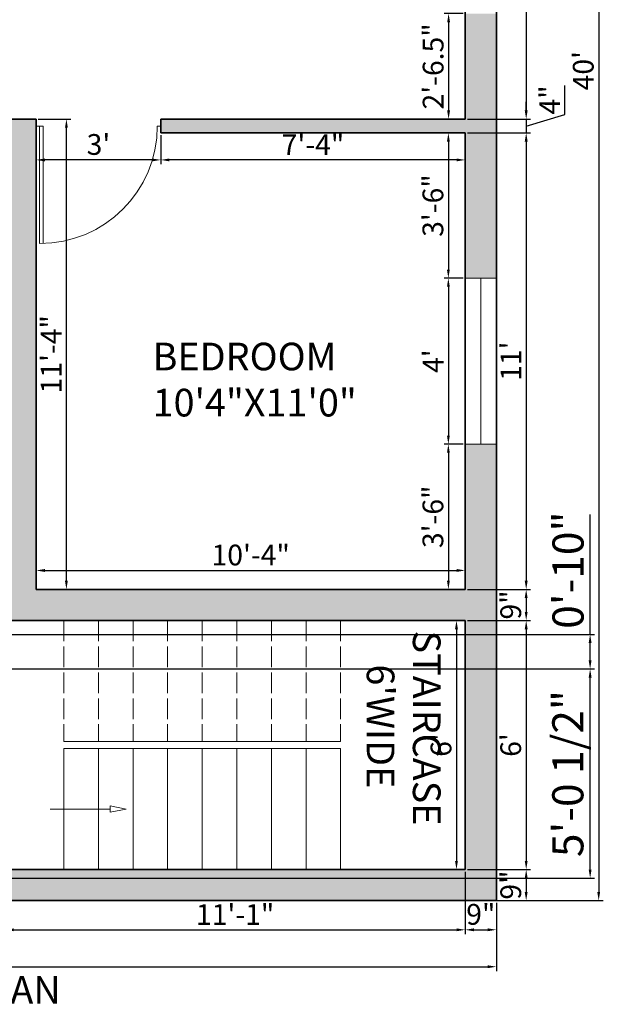
# Model space of a CAD drawing. Units: inches. Extents: x 3592 to 4861, y 1650 to 2243.
# Tile 28 of 30: x 4688 to 4861, y 1655 to 1940. Entities that reach past the tile are written whole.
import ezdxf

# ---------------------------------------------------------------- set-up
doc = ezdxf.new("R2010")
doc.units = ezdxf.units.IN
doc.linetypes.add('ACAD_ISO02W100', pattern=[15, 12, -3])
for name, color, linetype, lineweight in [('A-ANNO-DIMS', 2, 'Continuous', 13), ('A-ANNO-SYMB', 7, 'Continuous', 18), ('A-ANNO-TEXT', 7, 'Continuous', 25), ('A-AREA-IDEN', 7, 'Continuous', 18), ('A-DOOR', 3, 'Continuous', 20), ('A-FLOR-STRS', 7, 'Continuous', 18), ('A-FLOR-STRS-OVHD', 8, 'ACAD_ISO02W100', 13), ('A-GLAZ', 4, 'Continuous', 18), ('A-WALL', 7, 'Continuous', 35)]:
    doc.layers.add(name, color=color, linetype=linetype, lineweight=lineweight)
doc.layers.add('A-WALL-PATT', color=252, linetype='Continuous', lineweight=13, true_color=0x939598)
doc.styles.get("Standard").update_dxf_attribs({"font": 'arial.ttf'})
doc.dimstyles.new('ISO-25', dxfattribs={"dimtxt": 9, "dimasz": 2.5, "dimexe": 1.25, "dimexo": 0.625, "dimtad": 1, "dimlunit": 3, "dimtxsty": 'Standard', "dimcen": 2.5, "dimadec": 0, "dimazin": 0, "dimtfac": 1, "dimtmove": 0, "dimatfit": 3, "dimfxl": 1, "dimarcsym": 0})

# ---------------------------------------------------------------- blocks, each defined once
blk = doc.blocks.new('1')
for p, q in [((3628.27, 1890.86), (3628.27, 1924.86)), ((3629.27, 1890.86), (3629.27, 1924.86)), ((3627.27, 1890.86), (3629.27, 1890.86)), ((3662.27, 1890.86), (3663.27, 1890.86))]:
    blk.add_line(p, q)
blk.add_arc((3628.27, 1890.86), 34, 0, 90)
blk = doc.blocks.new('*D69')
at = {"layer": 'A-ANNO-DIMS', "color": 0, "lineweight": -2, "transparency": 16777216}
for p, q in [((4816.62, 1941.72), (4811.19, 1941.72)), ((4812.44, 1939.22), (4812.44, 1913.72)), ((4816.62, 1911.22), (4811.19, 1911.22))]:
    blk.add_line(p, q, dxfattribs=at)
at = {"layer": 'A-ANNO-DIMS', "color": 0, "transparency": 16777216}
for points in [[(4812.03, 1939.22), (4812.86, 1939.22), (4812.44, 1941.72)], [(4812.03, 1913.72), (4812.86, 1913.72), (4812.44, 1911.22)]]:
    blk.add_solid(points, dxfattribs=at)
at = {"layer": 'Defpoints', "color": 0, "transparency": 16777216}
for p in [(4817.25, 1941.72), (4812.44, 1911.22), (4817.25, 1911.22)]:
    blk.add_point(p, dxfattribs=at)
at = {"layer": 'A-ANNO-DIMS', "color": 0, "transparency": 16777216, "insert": (4808.75, 1926.47), "char_height": 6, "attachment_point": 5, "rotation": 90}
blk.add_mtext('2\'-6.5"', dxfattribs=at)
blk = doc.blocks.new('*D70')
at = {"layer": 'A-ANNO-DIMS', "color": 0, "lineweight": -2, "transparency": 16777216}
for p, q in [((4816.62, 1907.22), (4811.13, 1907.22)), ((4812.38, 1904.72), (4812.38, 1867.72)), ((4816.62, 1865.22), (4811.13, 1865.22))]:
    blk.add_line(p, q, dxfattribs=at)
at = {"layer": 'A-ANNO-DIMS', "color": 0, "transparency": 16777216}
for points in [[(4811.97, 1904.72), (4812.8, 1904.72), (4812.38, 1907.22)], [(4811.97, 1867.72), (4812.8, 1867.72), (4812.38, 1865.22)]]:
    blk.add_solid(points, dxfattribs=at)
at = {"layer": 'Defpoints', "color": 0, "transparency": 16777216}
for p in [(4817.25, 1907.22), (4812.38, 1865.22), (4817.25, 1865.22)]:
    blk.add_point(p, dxfattribs=at)
at = {"layer": 'A-ANNO-DIMS', "color": 0, "transparency": 16777216, "insert": (4808.69, 1886.22), "char_height": 6, "attachment_point": 5, "rotation": 90}
blk.add_mtext('3\'-6"', dxfattribs=at)
blk = doc.blocks.new('*D71')
at = {"layer": 'A-ANNO-DIMS', "color": 0, "lineweight": -2, "transparency": 16777216}
for p, q in [((4816.62, 1865.22), (4811.13, 1865.22)), ((4812.38, 1862.72), (4812.38, 1819.72)), ((4816.62, 1817.22), (4811.13, 1817.22))]:
    blk.add_line(p, q, dxfattribs=at)
at = {"layer": 'A-ANNO-DIMS', "color": 0, "transparency": 16777216}
for points in [[(4811.97, 1862.72), (4812.8, 1862.72), (4812.38, 1865.22)], [(4811.97, 1819.72), (4812.8, 1819.72), (4812.38, 1817.22)]]:
    blk.add_solid(points, dxfattribs=at)
at = {"layer": 'Defpoints', "color": 0, "transparency": 16777216}
for p in [(4817.25, 1865.22), (4812.38, 1817.22), (4817.25, 1817.22)]:
    blk.add_point(p, dxfattribs=at)
at = {"layer": 'A-ANNO-DIMS', "color": 0, "transparency": 16777216, "insert": (4808.76, 1841.22), "char_height": 6, "attachment_point": 5, "rotation": 90}
blk.add_mtext("4'", dxfattribs=at)
blk = doc.blocks.new('*D72')
at = {"layer": 'A-ANNO-DIMS', "color": 0, "lineweight": -2, "transparency": 16777216}
for p, q in [((4816.62, 1817.22), (4811.13, 1817.22)), ((4812.38, 1814.72), (4812.38, 1777.72)), ((4816.62, 1775.22), (4811.13, 1775.22))]:
    blk.add_line(p, q, dxfattribs=at)
at = {"layer": 'A-ANNO-DIMS', "color": 0, "transparency": 16777216}
for points in [[(4811.97, 1814.72), (4812.8, 1814.72), (4812.38, 1817.22)], [(4811.97, 1777.72), (4812.8, 1777.72), (4812.38, 1775.22)]]:
    blk.add_solid(points, dxfattribs=at)
at = {"layer": 'Defpoints', "color": 0, "transparency": 16777216}
for p in [(4817.25, 1817.22), (4812.38, 1775.22), (4817.25, 1775.22)]:
    blk.add_point(p, dxfattribs=at)
at = {"layer": 'A-ANNO-DIMS', "color": 0, "transparency": 16777216, "insert": (4808.69, 1796.22), "char_height": 6, "attachment_point": 5, "rotation": 90}
blk.add_mtext('3\'-6"', dxfattribs=at)
blk = doc.blocks.new('*D73')
at = {"layer": 'A-ANNO-DIMS', "color": 0, "lineweight": -2, "transparency": 16777216}
for p, q in [((4693.25, 1775.84), (4693.25, 1781.95)), ((4695.75, 1780.7), (4814.75, 1780.7)), ((4817.25, 1775.84), (4817.25, 1781.95))]:
    blk.add_line(p, q, dxfattribs=at)
at = {"layer": 'A-ANNO-DIMS', "color": 0, "transparency": 16777216}
for points in [[(4695.75, 1781.12), (4695.75, 1780.28), (4693.25, 1780.7)], [(4814.75, 1781.12), (4814.75, 1780.28), (4817.25, 1780.7)]]:
    blk.add_solid(points, dxfattribs=at)
at = {"layer": 'Defpoints', "color": 0, "transparency": 16777216}
for p in [(4817.25, 1780.7), (4693.25, 1775.22), (4817.25, 1775.22)]:
    blk.add_point(p, dxfattribs=at)
at = {"layer": 'A-ANNO-DIMS', "color": 0, "transparency": 16777216, "insert": (4755.25, 1784.39), "char_height": 6, "attachment_point": 5}
blk.add_mtext('10\'-4"', dxfattribs=at)
blk = doc.blocks.new('*D74')
at = {"layer": 'A-ANNO-DIMS', "color": 0, "lineweight": -2, "transparency": 16777216}
for p, q in [((4693.87, 1911.22), (4703.23, 1911.22)), ((4701.98, 1777.72), (4701.98, 1908.72)), ((4693.87, 1775.22), (4703.23, 1775.22))]:
    blk.add_line(p, q, dxfattribs=at)
at = {"layer": 'A-ANNO-DIMS', "color": 0, "transparency": 16777216}
for points in [[(4701.57, 1908.72), (4702.4, 1908.72), (4701.98, 1911.22)], [(4701.57, 1777.72), (4702.4, 1777.72), (4701.98, 1775.22)]]:
    blk.add_solid(points, dxfattribs=at)
at = {"layer": 'Defpoints', "color": 0, "transparency": 16777216}
for p in [(4693.25, 1911.22), (4701.98, 1911.22), (4693.25, 1775.22)]:
    blk.add_point(p, dxfattribs=at)
at = {"layer": 'A-ANNO-DIMS', "color": 0, "transparency": 16777216, "insert": (4698.35, 1843.22), "char_height": 6, "attachment_point": 5, "rotation": 90}
blk.add_mtext('11\'-4"', dxfattribs=at)
blk = doc.blocks.new('*D75')
at = {"layer": 'A-ANNO-DIMS', "color": 0, "lineweight": -2, "transparency": 16777216}
for p, q in [((4729.25, 1906.59), (4729.25, 1898.17)), ((4817.25, 1906.59), (4817.25, 1898.17)), ((4814.75, 1899.42), (4731.75, 1899.42))]:
    blk.add_line(p, q, dxfattribs=at)
at = {"layer": 'A-ANNO-DIMS', "color": 0, "transparency": 16777216}
for points in [[(4731.75, 1899.83), (4731.75, 1899), (4729.25, 1899.42)], [(4814.75, 1899.83), (4814.75, 1899), (4817.25, 1899.42)]]:
    blk.add_solid(points, dxfattribs=at)
at = {"layer": 'Defpoints', "color": 0, "transparency": 16777216}
for p in [(4729.25, 1907.22), (4817.25, 1907.22), (4729.25, 1899.42)]:
    blk.add_point(p, dxfattribs=at)
at = {"layer": 'A-ANNO-DIMS', "color": 0, "transparency": 16777216, "insert": (4773.25, 1903.04), "char_height": 6, "attachment_point": 5}
blk.add_mtext('7\'-4"', dxfattribs=at)
blk = doc.blocks.new('*D76')
at = {"layer": 'A-ANNO-DIMS', "color": 0, "lineweight": -2, "transparency": 16777216}
for p, q in [((4729.25, 1906.59), (4729.25, 1898.17)), ((4693.25, 1900.04), (4693.25, 1900.67)), ((4726.75, 1899.42), (4695.75, 1899.42))]:
    blk.add_line(p, q, dxfattribs=at)
at = {"layer": 'A-ANNO-DIMS', "color": 0, "transparency": 16777216}
for points in [[(4695.75, 1899.83), (4695.75, 1899), (4693.25, 1899.42)], [(4726.75, 1899.83), (4726.75, 1899), (4729.25, 1899.42)]]:
    blk.add_solid(points, dxfattribs=at)
at = {"layer": 'Defpoints', "color": 0, "transparency": 16777216}
for p in [(4729.25, 1907.22), (4693.25, 1899.42), (4693.25, 1899.42)]:
    blk.add_point(p, dxfattribs=at)
at = {"layer": 'A-ANNO-DIMS', "color": 0, "transparency": 16777216, "insert": (4711.25, 1903.11), "char_height": 6, "attachment_point": 5}
blk.add_mtext("3'", dxfattribs=at)
blk = doc.blocks.new('*D98')
at = {"layer": 'A-ANNO-DIMS', "color": 0, "lineweight": -2, "transparency": 16777216}
for p, q in [((4817.25, 1693.59), (4817.25, 1675.54)), ((4684.25, 1684.59), (4684.25, 1675.54)), ((4686.75, 1676.79), (4814.75, 1676.79))]:
    blk.add_line(p, q, dxfattribs=at)
at = {"layer": 'A-ANNO-DIMS', "color": 0, "transparency": 16777216}
for points in [[(4686.75, 1677.2), (4686.75, 1676.37), (4684.25, 1676.79)], [(4814.75, 1677.2), (4814.75, 1676.37), (4817.25, 1676.79)]]:
    blk.add_solid(points, dxfattribs=at)
at = {"layer": 'Defpoints', "color": 0, "transparency": 16777216}
for p in [(4817.25, 1694.22), (4684.25, 1685.22), (4817.25, 1676.79)]:
    blk.add_point(p, dxfattribs=at)
at = {"layer": 'A-ANNO-DIMS', "color": 0, "transparency": 16777216, "insert": (4750.75, 1680.42), "char_height": 6, "attachment_point": 5}
blk.add_mtext('11\'-1"', dxfattribs=at)
blk = doc.blocks.new('*D99')
at = {"layer": 'A-ANNO-DIMS', "color": 0, "lineweight": -2, "transparency": 16777216}
for p, q in [((4817.25, 1693.59), (4817.25, 1675.54)), ((4826.25, 1684.59), (4826.25, 1675.54)), ((4819.75, 1676.79), (4823.75, 1676.79))]:
    blk.add_line(p, q, dxfattribs=at)
at = {"layer": 'A-ANNO-DIMS', "color": 0, "transparency": 16777216}
for points in [[(4819.75, 1677.2), (4819.75, 1676.37), (4817.25, 1676.79)], [(4823.75, 1677.2), (4823.75, 1676.37), (4826.25, 1676.79)]]:
    blk.add_solid(points, dxfattribs=at)
at = {"layer": 'Defpoints', "color": 0, "transparency": 16777216}
for p in [(4817.25, 1694.22), (4826.25, 1685.22), (4826.25, 1676.79)]:
    blk.add_point(p, dxfattribs=at)
at = {"layer": 'A-ANNO-DIMS', "color": 0, "transparency": 16777216, "insert": (4821.75, 1680.48), "char_height": 6, "attachment_point": 5}
blk.add_mtext('9"', dxfattribs=at)
blk = doc.blocks.new('*D121')
at = {"layer": 'A-ANNO-DIMS', "color": 0, "lineweight": -2, "transparency": 16777216}
for p, q in [((4817.87, 2020.22), (4836.12, 2020.22)), ((4834.87, 2017.72), (4834.87, 1913.72)), ((4817.87, 1911.22), (4836.12, 1911.22))]:
    blk.add_line(p, q, dxfattribs=at)
at = {"layer": 'A-ANNO-DIMS', "color": 0, "transparency": 16777216}
for points in [[(4834.45, 2017.72), (4835.29, 2017.72), (4834.87, 2020.22)], [(4834.45, 1913.72), (4835.29, 1913.72), (4834.87, 1911.22)]]:
    blk.add_solid(points, dxfattribs=at)
at = {"layer": 'Defpoints', "color": 0, "transparency": 16777216}
for p in [(4817.25, 2020.22), (4817.25, 1911.22), (4834.87, 1911.22)]:
    blk.add_point(p, dxfattribs=at)
at = {"layer": 'A-ANNO-DIMS', "color": 0, "transparency": 16777216, "insert": (4831.18, 1965.72), "char_height": 6, "attachment_point": 5, "rotation": 90}
blk.add_mtext('9\'-1"', dxfattribs=at)
blk = doc.blocks.new('*D122')
at = {"layer": 'A-ANNO-DIMS', "color": 0, "lineweight": -2, "transparency": 16777216}
for p, q in [((4846.06, 1912.58), (4846.06, 1920.96)), ((4834.87, 1913.72), (4834.87, 1916.22)), ((4817.87, 1911.22), (4836.12, 1911.22)), ((4834.87, 1909.22), (4846.06, 1912.58)), ((4834.87, 1911.22), (4834.87, 1907.22)), ((4834.87, 1911.22), (4834.87, 1907.22)), ((4817.87, 1907.22), (4836.12, 1907.22)), ((4834.87, 1904.72), (4834.87, 1902.22))]:
    blk.add_line(p, q, dxfattribs=at)
at = {"layer": 'A-ANNO-DIMS', "color": 0, "transparency": 16777216}
for points in [[(4834.45, 1913.72), (4835.29, 1913.72), (4834.87, 1911.22)], [(4834.45, 1904.72), (4835.29, 1904.72), (4834.87, 1907.22)]]:
    blk.add_solid(points, dxfattribs=at)
at = {"layer": 'Defpoints', "color": 0, "transparency": 16777216}
for p in [(4817.25, 1911.22), (4817.25, 1907.22), (4834.87, 1907.22)]:
    blk.add_point(p, dxfattribs=at)
at = {"layer": 'A-ANNO-DIMS', "color": 0, "transparency": 16777216, "insert": (4842.43, 1916.77), "char_height": 6, "attachment_point": 5, "rotation": 90}
blk.add_mtext('4"', dxfattribs=at)
blk = doc.blocks.new('*D123')
at = {"layer": 'A-ANNO-DIMS', "color": 0, "lineweight": -2, "transparency": 16777216}
for p, q in [((4817.87, 1907.22), (4836.12, 1907.22)), ((4834.87, 1904.72), (4834.87, 1777.72)), ((4817.87, 1775.22), (4836.12, 1775.22))]:
    blk.add_line(p, q, dxfattribs=at)
at = {"layer": 'A-ANNO-DIMS', "color": 0, "transparency": 16777216}
for points in [[(4834.45, 1904.72), (4835.29, 1904.72), (4834.87, 1907.22)], [(4834.45, 1777.72), (4835.29, 1777.72), (4834.87, 1775.22)]]:
    blk.add_solid(points, dxfattribs=at)
at = {"layer": 'Defpoints', "color": 0, "transparency": 16777216}
for p in [(4817.25, 1907.22), (4817.25, 1775.22), (4834.87, 1775.22)]:
    blk.add_point(p, dxfattribs=at)
at = {"layer": 'A-ANNO-DIMS', "color": 0, "transparency": 16777216, "insert": (4831.23, 1841.22), "char_height": 6, "attachment_point": 5, "rotation": 90}
blk.add_mtext("11'", dxfattribs=at)
blk = doc.blocks.new('*D124')
at = {"layer": 'A-ANNO-DIMS', "color": 0, "lineweight": -2, "transparency": 16777216}
for p, q in [((4817.87, 1775.22), (4836.12, 1775.22)), ((4834.87, 1772.72), (4834.87, 1768.72)), ((4817.87, 1766.22), (4836.12, 1766.22))]:
    blk.add_line(p, q, dxfattribs=at)
at = {"layer": 'A-ANNO-DIMS', "color": 0, "transparency": 16777216}
for points in [[(4834.45, 1772.72), (4835.29, 1772.72), (4834.87, 1775.22)], [(4834.45, 1768.72), (4835.29, 1768.72), (4834.87, 1766.22)]]:
    blk.add_solid(points, dxfattribs=at)
at = {"layer": 'Defpoints', "color": 0, "transparency": 16777216}
for p in [(4817.25, 1775.22), (4817.25, 1766.22), (4834.87, 1766.22)]:
    blk.add_point(p, dxfattribs=at)
at = {"layer": 'A-ANNO-DIMS', "color": 0, "transparency": 16777216, "insert": (4831.18, 1770.72), "char_height": 6, "attachment_point": 5, "rotation": 90}
blk.add_mtext('9"', dxfattribs=at)
blk = doc.blocks.new('*D125')
at = {"layer": 'A-ANNO-DIMS', "color": 0, "lineweight": -2, "transparency": 16777216}
for p, q in [((4817.87, 1766.22), (4836.12, 1766.22)), ((4834.87, 1763.72), (4834.87, 1696.72)), ((4817.87, 1694.22), (4836.12, 1694.22))]:
    blk.add_line(p, q, dxfattribs=at)
at = {"layer": 'A-ANNO-DIMS', "color": 0, "transparency": 16777216}
for points in [[(4834.45, 1763.72), (4835.29, 1763.72), (4834.87, 1766.22)], [(4834.45, 1696.72), (4835.29, 1696.72), (4834.87, 1694.22)]]:
    blk.add_solid(points, dxfattribs=at)
at = {"layer": 'Defpoints', "color": 0, "transparency": 16777216}
for p in [(4817.25, 1766.22), (4817.25, 1694.22), (4834.87, 1694.22)]:
    blk.add_point(p, dxfattribs=at)
at = {"layer": 'A-ANNO-DIMS', "color": 0, "transparency": 16777216, "insert": (4831.18, 1730.22), "char_height": 6, "attachment_point": 5, "rotation": 90}
blk.add_mtext("6'", dxfattribs=at)
blk = doc.blocks.new('*D126')
at = {"layer": 'A-ANNO-DIMS', "color": 0, "lineweight": -2, "transparency": 16777216}
for p, q in [((4817.87, 1694.22), (4836.12, 1694.22)), ((4834.87, 1691.72), (4834.87, 1687.72)), ((4817.87, 1685.22), (4836.12, 1685.22))]:
    blk.add_line(p, q, dxfattribs=at)
at = {"layer": 'A-ANNO-DIMS', "color": 0, "transparency": 16777216}
for points in [[(4834.45, 1691.72), (4835.29, 1691.72), (4834.87, 1694.22)], [(4834.45, 1687.72), (4835.29, 1687.72), (4834.87, 1685.22)]]:
    blk.add_solid(points, dxfattribs=at)
at = {"layer": 'Defpoints', "color": 0, "transparency": 16777216}
for p in [(4817.25, 1694.22), (4817.25, 1685.22), (4834.87, 1685.22)]:
    blk.add_point(p, dxfattribs=at)
at = {"layer": 'A-ANNO-DIMS', "color": 0, "transparency": 16777216, "insert": (4831.18, 1689.72), "char_height": 6, "attachment_point": 5, "rotation": 90}
blk.add_mtext('9"', dxfattribs=at)
blk = doc.blocks.new('*D127')
at = {"layer": 'A-ANNO-DIMS', "color": 0, "lineweight": -2, "transparency": 16777216}
for p, q in [((4466.25, 1684.59), (4466.25, 1664.86)), ((4826.25, 1684.59), (4826.25, 1664.86)), ((4468.75, 1666.11), (4823.75, 1666.11))]:
    blk.add_line(p, q, dxfattribs=at)
at = {"layer": 'A-ANNO-DIMS', "color": 0, "transparency": 16777216}
for points in [[(4468.75, 1666.53), (4468.75, 1665.69), (4466.25, 1666.11)], [(4823.75, 1666.53), (4823.75, 1665.69), (4826.25, 1666.11)]]:
    blk.add_solid(points, dxfattribs=at)
at = {"layer": 'Defpoints', "color": 0, "transparency": 16777216}
for p in [(4466.25, 1685.22), (4826.25, 1685.22), (4826.25, 1666.11)]:
    blk.add_point(p, dxfattribs=at)
at = {"layer": 'A-ANNO-DIMS', "color": 0, "transparency": 16777216, "insert": (4646.25, 1669.8), "char_height": 6, "attachment_point": 5}
blk.add_mtext("30'", dxfattribs=at)
blk = doc.blocks.new('*D129')
at = {"layer": 'A-ANNO-DIMS', "color": 0, "lineweight": -2, "transparency": 16777216}
for p, q in [((4816.62, 1766.22), (4813.47, 1766.22)), ((4814.72, 1763.72), (4814.72, 1696.72)), ((4816.62, 1694.22), (4813.47, 1694.22))]:
    blk.add_line(p, q, dxfattribs=at)
at = {"layer": 'A-ANNO-DIMS', "color": 0, "transparency": 16777216}
for points in [[(4814.3, 1763.72), (4815.14, 1763.72), (4814.72, 1766.22)], [(4814.3, 1696.72), (4815.14, 1696.72), (4814.72, 1694.22)]]:
    blk.add_solid(points, dxfattribs=at)
at = {"layer": 'Defpoints', "color": 0, "transparency": 16777216}
for p in [(4817.25, 1766.22), (4814.72, 1694.22), (4817.25, 1694.22)]:
    blk.add_point(p, dxfattribs=at)
at = {"layer": 'A-ANNO-DIMS', "color": 0, "transparency": 16777216, "insert": (4811.03, 1730.22), "char_height": 6, "attachment_point": 5, "rotation": 90}
blk.add_mtext("6'", dxfattribs=at)
blk = doc.blocks.new('*D133')
at = {"layer": 'A-ANNO-DIMS', "color": 0, "lineweight": -2, "transparency": 16777216}
for p, q in [((4826.87, 2165.22), (4857.08, 2165.22)), ((4855.83, 2162.72), (4855.83, 1687.72)), ((4826.87, 1685.22), (4857.08, 1685.22))]:
    blk.add_line(p, q, dxfattribs=at)
at = {"layer": 'A-ANNO-DIMS', "color": 0, "transparency": 16777216}
for points in [[(4855.41, 2162.72), (4856.24, 2162.72), (4855.83, 2165.22)], [(4855.41, 1687.72), (4856.24, 1687.72), (4855.83, 1685.22)]]:
    blk.add_solid(points, dxfattribs=at)
at = {"layer": 'Defpoints', "color": 0, "transparency": 16777216}
for p in [(4826.25, 2165.22), (4826.25, 1685.22), (4855.83, 1685.22)]:
    blk.add_point(p, dxfattribs=at)
at = {"layer": 'A-ANNO-DIMS', "color": 0, "transparency": 16777216, "insert": (4852.14, 1925.22), "char_height": 6, "attachment_point": 5, "rotation": 90}
blk.add_mtext("40'", dxfattribs=at)
blk = doc.blocks.new('ARROW-STAIR-DIRECTION')
blk.add_line((0, 0.94), (17.38, 0.94))
blk.add_lwpolyline([(22.04, 0.94), (17.38, 1.89), (17.38, 0)], close=True)
blk = doc.blocks.new('STAIR-LOWER-RUN')
for p, q in [((0, 35), (80, 35)), ((0, 35), (0, 0)), ((10, 35), (10, 0)), ((20, 35), (20, 0)), ((30, 35), (30, 0)), ((40, 35), (40, 0)), ((50, 35), (50, 0)), ((60, 35), (60, 0)), ((70, 35), (70, 0)), ((80, 35), (80, 0))]:
    blk.add_line(p, q)
blk = doc.blocks.new('STAIR-UPPER-RUN')
at = {"ltscale": 0.5}
for p, q in [((0, 35), (0, 0)), ((10, 35), (10, 0)), ((20, 35), (20, 0)), ((30, 35), (30, 0)), ((40, 35), (40, 0)), ((50, 35), (50, 0)), ((60, 35), (60, 0)), ((70, 35), (70, 0)), ((80, 35), (80, 0))]:
    blk.add_line(p, q, dxfattribs=at)
blk = doc.blocks.new('*D183')
at = {"layer": 'A-ANNO-DIMS', "color": 0, "lineweight": -2, "transparency": 16777216}
for p, q in [((4853.35, 1762.22), (4853.35, 1796.89)), ((4580.87, 1762.22), (4854.6, 1762.22)), ((4853.35, 1754.72), (4853.35, 1759.72)), ((4580.87, 1752.22), (4854.6, 1752.22))]:
    blk.add_line(p, q, dxfattribs=at)
at = {"layer": 'A-ANNO-DIMS', "color": 0, "transparency": 16777216}
for points in [[(4852.93, 1759.72), (4853.77, 1759.72), (4853.35, 1762.22)], [(4852.93, 1754.72), (4853.77, 1754.72), (4853.35, 1752.22)]]:
    blk.add_solid(points, dxfattribs=at)
at = {"layer": 'Defpoints', "color": 0, "transparency": 16777216}
for p in [(4580.25, 1762.22), (4853.35, 1762.22), (4580.25, 1752.22)]:
    blk.add_point(p, dxfattribs=at)
at = {"layer": 'A-ANNO-DIMS', "color": 0, "transparency": 16777216, "insert": (4848.13, 1780.8), "char_height": 9, "attachment_point": 5, "rotation": 90}
blk.add_mtext('0\'-10"', dxfattribs=at)
blk = doc.blocks.new('*D184')
at = {"layer": 'A-ANNO-DIMS', "color": 0, "lineweight": -2, "transparency": 16777216}
for p, q in [((4580.87, 1752.22), (4854.6, 1752.22)), ((4853.35, 1694.22), (4853.35, 1749.72)), ((4580.87, 1691.72), (4854.6, 1691.72))]:
    blk.add_line(p, q, dxfattribs=at)
at = {"layer": 'A-ANNO-DIMS', "color": 0, "transparency": 16777216}
for points in [[(4852.93, 1749.72), (4853.77, 1749.72), (4853.35, 1752.22)], [(4852.93, 1694.22), (4853.77, 1694.22), (4853.35, 1691.72)]]:
    blk.add_solid(points, dxfattribs=at)
at = {"layer": 'Defpoints', "color": 0, "transparency": 16777216}
for p in [(4580.25, 1752.22), (4853.35, 1752.22), (4580.25, 1691.72)]:
    blk.add_point(p, dxfattribs=at)
at = {"layer": 'A-ANNO-DIMS', "color": 0, "transparency": 16777216, "insert": (4848.07, 1721.97), "char_height": 9, "attachment_point": 5, "rotation": 90}
blk.add_mtext('5\'-0 1/2"', dxfattribs=at)

msp = doc.modelspace()

# ---------------------------------------------------------------- hatches: boundary and pattern name
at = {"layer": 'A-WALL-PATT'}
h = msp.add_hatch(color=256, dxfattribs=at)
h.dxf.hatch_style = 1
h.paths.add_polyline_path([(4466.25, 2165.219), (4466.25, 1993.219), (4475.25, 1993.219), (4475.25, 2156.219), (4619.25, 2156.219), (4619.25, 2150.219), (4623.25, 2150.219), (4623.25, 2156.219), (4684.25, 2156.219), (4684.25, 2150.219), (4693.25, 2150.219), (4693.25, 2156.219), (4817.25, 2156.219), (4817.25, 2114.219), (4826.25, 2114.219), (4826.25, 2165.219)])
h.paths.add_polyline_path([(4623.25, 2096.219), (4623.25, 2102.219), (4619.25, 2102.219), (4619.25, 2020.219), (4623.25, 2020.219), (4623.25, 2087.219), (4684.25, 2087.219), (4684.25, 2020.219), (4734.25, 2020.219), (4734.25, 2024.219), (4693.25, 2024.219), (4693.25, 2102.219), (4684.25, 2102.219), (4684.25, 2096.219)], flags=17)
h.paths.add_polyline_path([(4817.25, 2024.219), (4776.25, 2024.219), (4776.25, 2020.219), (4817.25, 2020.219), (4817.25, 1989.719), (4826.25, 1989.719), (4826.25, 2066.219), (4817.25, 2066.219)])
h.paths.add_polyline_path([(4817.25, 1865.219), (4826.25, 1865.219), (4826.25, 1941.719), (4817.25, 1941.719), (4817.25, 1911.219), (4729.25, 1911.219), (4729.25, 1907.219), (4817.25, 1907.219)])
h.paths.add_polyline_path([(4826.25, 1817.219), (4817.25, 1817.219), (4817.25, 1775.219), (4693.25, 1775.219), (4693.25, 1911.219), (4684.25, 1911.219), (4684.25, 1817.219), (4648.75, 1817.219), (4648.75, 1808.219), (4684.25, 1808.219), (4684.25, 1766.219), (4817.25, 1766.219), (4817.25, 1694.219), (4684.25, 1694.219), (4684.25, 1685.219), (4826.25, 1685.219)])
h.paths.add_polyline_path([(4505.25, 1817.219), (4505.25, 1808.219), (4606.75, 1808.219), (4606.75, 1817.219)])
h.paths.add_polyline_path([(4539.25, 1856.219), (4539.25, 2020.219), (4583.25, 2020.219), (4583.25, 2024.219), (4505.25, 2024.219), (4505.25, 2020.219), (4535.25, 2020.219), (4535.25, 1942.219), (4475.25, 1942.219), (4475.25, 1969.219), (4466.25, 1969.219), (4466.25, 1911.219), (4475.25, 1911.219), (4475.25, 1938.219), (4535.25, 1938.219), (4535.25, 1860.219), (4505.25, 1860.219), (4505.25, 1856.219)])
h.paths.add_polyline_path([(4475.25, 1887.219), (4466.25, 1887.219), (4466.25, 1685.219), (4580.25, 1685.219), (4580.25, 1715.219), (4571.25, 1715.219), (4571.25, 1694.219), (4475.25, 1694.219)])
h.paths.add_polyline_path([(4571.25, 1751.219), (4580.25, 1751.219), (4580.25, 1772.219), (4571.25, 1772.219)], flags=17)

# ---------------------------------------------------------------- linework, layer by layer
at = {"layer": 'A-FLOR-STRS'}
msp.add_line((4701.25, 1731.219), (4781.25, 1731.219), dxfattribs=at)
at = {"layer": 'A-GLAZ'}
for p, q in [((4817.25, 1865.219), (4826.25, 1865.219)), ((4821.75, 1865.219), (4821.75, 1817.219)), ((4817.25, 1817.219), (4826.25, 1817.219))]:
    msp.add_line(p, q, dxfattribs=at)
at = {"layer": 'A-WALL'}
for p, q in [((4826.25, 2165.219), (4826.25, 1685.219)), ((4817.25, 2020.219), (4817.25, 1911.219)), ((4693.25, 1911.219), (4684.25, 1911.219)), ((4693.25, 1911.219), (4693.25, 1775.219)), ((4729.25, 1911.219), (4729.25, 1907.219)), ((4817.25, 1911.219), (4729.25, 1911.219)), ((4817.25, 1907.219), (4729.25, 1907.219)), ((4817.25, 1907.219), (4817.25, 1775.219)), ((4817.25, 1775.219), (4693.25, 1775.219)), ((4817.25, 1766.219), (4684.25, 1766.219)), ((4817.25, 1766.219), (4817.25, 1694.219)), ((4817.25, 1694.219), (4684.25, 1694.219)), ((4826.25, 1685.219), (4684.25, 1685.219))]:
    msp.add_line(p, q, dxfattribs=at)

# ---------------------------------------------------------------- block references
at = {"layer": 'A-ANNO-SYMB'}
msp.add_blockref('ARROW-STAIR-DIRECTION', (4697.257, 1710.776), dxfattribs=at)
at = {"layer": 'A-DOOR', "xscale": -1, "rotation": 180}
msp.add_blockref('1', (1065.982, 3800.083), dxfattribs=at)
at = {"layer": 'A-FLOR-STRS'}
msp.add_blockref('STAIR-LOWER-RUN', (4701.249, 1694.219), dxfattribs=at)
at = {"layer": 'A-FLOR-STRS-OVHD'}
msp.add_blockref('STAIR-UPPER-RUN', (4701.249, 1731.219), dxfattribs=at)

# ---------------------------------------------------------------- texts
at = {"layer": 'A-ANNO-TEXT', "insert": (4587.182, 1663.381), "char_height": 8, "attachment_point": 1}
msp.add_mtext_dynamic_manual_height_columns('GROUND FLOOR PLAN', width=131.60551, gutter_width=12.5, heights=[0], dxfattribs=at)
at = {"layer": 'A-AREA-IDEN', "insert": (4726.898, 1846.565), "char_height": 8, "attachment_point": 1}
msp.add_mtext_dynamic_manual_height_columns('BEDROOM\\P10\'4"X11\'0"', width=121.44943, gutter_width=12.5, heights=[0], dxfattribs=at)
at = {"layer": 'A-AREA-IDEN', "insert": (4810.122, 1763.303), "char_height": 8, "attachment_point": 1, "rotation": 270}
msp.add_mtext_dynamic_manual_height_columns("STAIRCASE\\P    6'WIDE", width=121.44943, gutter_width=12.5, heights=[0], dxfattribs=at)

# ---------------------------------------------------------------- dimensions: what is measured, and where the dimension line sits
at = {"layer": 'A-ANNO-DIMS'}
for base, p1, p2, override, picture, middle in [((4855.826, 1685.219), (4826.25, 2165.219), (4826.25, 1685.219), {"dimtxt": 6, "dimclrd": 0, "dimclre": 0, "dimclrt": 0}, '*D133', (4852.137, 1925.219)), ((4834.871, 1911.219), (4817.25, 2020.219), (4817.25, 1911.219), {"dimtxt": 6, "dimclrd": 0, "dimclre": 0, "dimclrt": 0, "dimtmove": 1}, '*D121', (4831.182, 1965.719)), ((4812.443, 1911.219), (4817.25, 1941.719), (4817.25, 1911.219), {"dimtxt": 6, "dimclrd": 0, "dimclre": 0, "dimclrt": 0, "dimtmove": 1}, '*D69', (4808.755, 1926.469)), ((4834.871, 1907.219), (4817.25, 1911.219), (4817.25, 1907.219), {"dimtxt": 6, "dimclrd": 0, "dimclre": 0, "dimclrt": 0, "dimtmove": 1}, '*D122', (4842.433, 1913.2)), ((4701.983, 1911.219), (4693.25, 1775.219), (4693.25, 1911.219), {"dimtxt": 6, "dimclrd": 0, "dimclre": 0, "dimclrt": 0}, '*D74', (4698.346, 1843.219)), ((4812.384, 1865.219), (4817.25, 1907.219), (4817.25, 1865.219), {"dimtxt": 6, "dimclrd": 0, "dimclre": 0, "dimclrt": 0}, '*D70', (4808.693, 1886.219)), ((4834.871, 1775.219), (4817.25, 1907.219), (4817.25, 1775.219), {"dimtxt": 6, "dimclrd": 0, "dimclre": 0, "dimclrt": 0, "dimtmove": 1}, '*D123', (4831.234, 1841.219)), ((4812.384, 1817.219), (4817.25, 1865.219), (4817.25, 1817.219), {"dimtxt": 6, "dimclrd": 0, "dimclre": 0, "dimclrt": 0, "dimtmove": 1}, '*D71', (4808.759, 1841.219)), ((4812.384, 1775.219), (4817.25, 1817.219), (4817.25, 1775.219), {"dimtxt": 6, "dimclrd": 0, "dimclre": 0, "dimclrt": 0, "dimtmove": 1}, '*D72', (4808.693, 1796.219)), ((4853.35, 1762.219), (4580.25, 1752.219), (4580.25, 1762.219), {"dimdec": 1, "dimlfac": 1, "dimrnd": 0, "dimzin": 1, "dimdsep": 46, "dimlunit": 4, "dimfrac": 2}, '*D183', (4848.13, 1780.802)), ((4834.871, 1766.219), (4817.25, 1775.219), (4817.25, 1766.219), {"dimtxt": 6, "dimclrd": 0, "dimclre": 0, "dimclrt": 0, "dimtmove": 1}, '*D124', (4831.182, 1770.719)), ((4814.721, 1694.219), (4817.25, 1766.219), (4817.25, 1694.219), {"dimtxt": 6, "dimclrd": 0, "dimclre": 0, "dimclrt": 0}, '*D129', (4811.032, 1730.219)), ((4834.871, 1694.219), (4817.25, 1766.219), (4817.25, 1694.219), {"dimtxt": 6, "dimclrd": 0, "dimclre": 0, "dimclrt": 0, "dimtmove": 1}, '*D125', (4831.182, 1730.219)), ((4853.35, 1752.219), (4580.25, 1691.719), (4580.25, 1752.219), {"dimdec": 1, "dimlfac": 1, "dimrnd": 0, "dimzin": 1, "dimdsep": 46, "dimlunit": 4, "dimfrac": 2}, '*D184', (4848.071, 1721.969)), ((4834.871, 1685.219), (4817.25, 1694.219), (4817.25, 1685.219), {"dimtxt": 6, "dimclrd": 0, "dimclre": 0, "dimclrt": 0, "dimtmove": 1}, '*D126', (4831.182, 1689.719))]:
    dim = msp.add_linear_dim(base=base, p1=p1, p2=p2, angle=90, dimstyle='ISO-25', override=override, dxfattribs=at)
    dim.commit()
    dim.dimension.update_dxf_attribs({"geometry": picture, "text_midpoint": middle})
for base, p1, p2, override, picture, middle in [((4693.25, 1899.415), (4729.25, 1907.219), (4693.25, 1899.415), {"dimtxt": 6, "dimclrd": 0, "dimclre": 0, "dimclrt": 0, "dimtmove": 1}, '*D76', (4711.25, 1903.106)), ((4729.25, 1899.415), (4817.25, 1907.219), (4729.25, 1907.219), {"dimtxt": 6, "dimclrd": 0, "dimclre": 0, "dimclrt": 0}, '*D75', (4773.25, 1903.04)), ((4817.25, 1780.699), (4693.25, 1775.219), (4817.25, 1775.219), {"dimtxt": 6, "dimclrd": 0, "dimclre": 0, "dimclrt": 0}, '*D73', (4755.25, 1784.388)), ((4817.25, 1676.787), (4684.25, 1685.219), (4817.25, 1694.219), {"dimtxt": 6, "dimclrd": 0, "dimclre": 0, "dimclrt": 0, "dimtmove": 1}, '*D98', (4750.75, 1680.424)), ((4826.25, 1676.787), (4817.25, 1694.219), (4826.25, 1685.219), {"dimtxt": 6, "dimclrd": 0, "dimclre": 0, "dimclrt": 0, "dimtmove": 1}, '*D99', (4821.75, 1680.476)), ((4826.25, 1666.109), (4466.25, 1685.219), (4826.25, 1685.219), {"dimtxt": 6, "dimclrd": 0, "dimclre": 0, "dimclrt": 0}, '*D127', (4646.25, 1669.799))]:
    dim = msp.add_linear_dim(base=base, p1=p1, p2=p2, dimstyle='ISO-25', override=override, dxfattribs=at)
    dim.commit()
    dim.dimension.update_dxf_attribs({"geometry": picture, "text_midpoint": middle})

doc.saveas('drawing.dxf')
